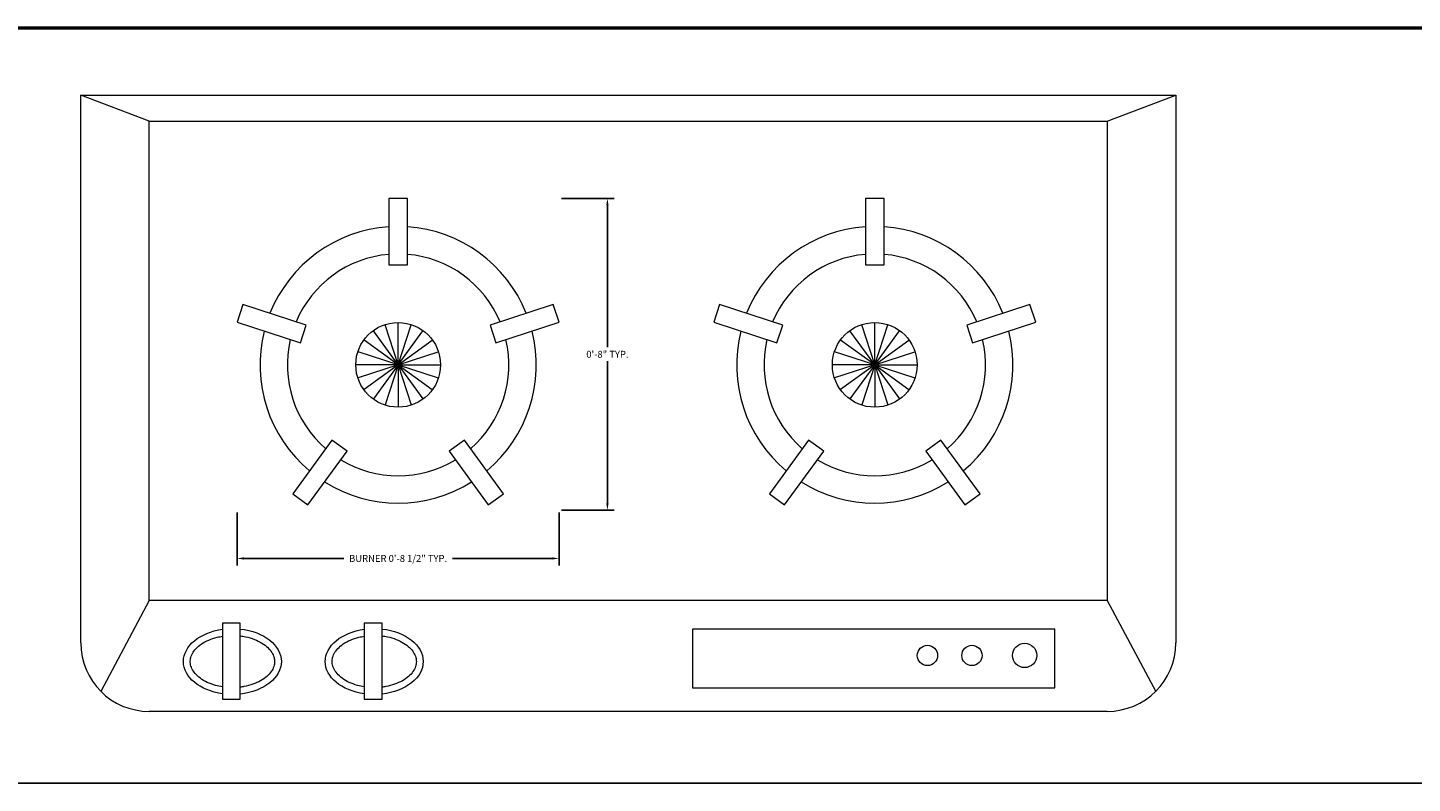
# Model space of a CAD drawing. Units: inches. Extents: x -173 to 545, y -746 to 104.
# Tile 28 of 32: x 189 to 225, y -12 to 8. Entities that reach past the tile are written whole.
import ezdxf

# ---------------------------------------------------------------- set-up
doc = ezdxf.new("R2010")
doc.units = ezdxf.units.IN
doc.header["$MEASUREMENT"] = 0
for name, color, linetype, lineweight in [('A-ANNO-DIMS', 2, 'Continuous', 18), ('A-EQPM', 8, 'Continuous', 18), ('A-FLOR-CASE', 9, 'Continuous', 25), ('A-WALL', 7, 'Continuous', 50)]:
    doc.layers.add(name, color=color, linetype=linetype, lineweight=lineweight)
doc.styles.get("Standard").update_dxf_attribs({"font": 'arial.ttf'})
doc.dimstyles.get("Standard").update_dxf_attribs({"dimtxt": 0.18, "dimasz": 0.18, "dimexe": 0.18, "dimexo": 0.0625, "dimgap": 0.09, "dimtad": 0, "dimtih": 1, "dimtoh": 1, "dimdec": 0, "dimzin": 0, "dimdsep": 46, "dimlunit": 3, "dimtxsty": 'Standard', "dimcen": 0.09, "dimadec": 0, "dimazin": 0, "dimtfac": 1, "dimtdec": 0, "dimtofl": 0, "dimtmove": 0, "dimatfit": 3, "dimfxl": 1, "dimtolj": 1, "dimtzin": 0, "dimarcsym": 0})

# ---------------------------------------------------------------- blocks, each defined once
blk = doc.blocks.new('HOB-28-BURNER')
for p, q in [((4.43, 7.964), (3.944, 7.964)), ((3.944, 7.964), (3.944, 6.235)), ((4.43, 6.235), (4.43, 7.964)), ((3.944, 6.235), (4.43, 6.235)), ((0.151, 5.207), (0, 4.745)), ((1.795, 4.673), (0.151, 5.207)), ((8.223, 5.207), (6.579, 4.673)), ((8.374, 4.745), (8.223, 5.207)), ((0, 4.745), (1.644, 4.211)), ((4.187, 3.64), (3.848, 4.683)), ((4.187, 3.64), (4.187, 4.737)), ((4.187, 3.64), (4.526, 4.683)), ((6.73, 4.211), (8.374, 4.745)), ((1.644, 4.211), (1.795, 4.673)), ((4.187, 3.64), (3.543, 4.527)), ((4.187, 3.64), (4.831, 4.527)), ((6.579, 4.673), (6.73, 4.211)), ((4.187, 3.64), (3.144, 3.979)), ((4.187, 3.64), (3.3, 4.285)), ((4.187, 3.64), (5.074, 4.285)), ((4.187, 3.64), (5.23, 3.979)), ((4.187, 3.64), (3.091, 3.64)), ((4.187, 3.64), (3.144, 3.302)), ((4.187, 3.64), (3.3, 2.996)), ((4.187, 3.64), (3.543, 2.754)), ((4.187, 3.64), (3.848, 2.598)), ((4.187, 3.64), (4.187, 2.544)), ((4.187, 3.64), (4.526, 2.598)), ((4.187, 3.64), (4.831, 2.754)), ((4.187, 3.64), (5.074, 2.996)), ((4.187, 3.64), (5.23, 3.302)), ((4.187, 3.64), (5.283, 3.64)), ((2.465, 1.684), (1.449, 0.286)), ((2.859, 1.399), (2.465, 1.684)), ((5.909, 1.684), (5.515, 1.399)), ((6.925, 0.286), (5.909, 1.684)), ((1.842, 0), (2.859, 1.399)), ((5.515, 1.399), (6.532, 0)), ((1.449, 0.286), (1.842, 0)), ((6.532, 0), (6.925, 0.286))]:
    blk.add_line(p, q)
blk.add_circle((4.187, 3.64), 1.101)
for radius, start, end in [(3.593, 93.8765, 158.1235), (3.593, 21.8765, 86.1235), (2.881, 94.8365, 157.1635), (2.881, 22.8365, 85.1635), (3.593, 165.8765, 230.1235), (3.593, 309.8765, 14.1235), (2.881, 166.8365, 229.1635), (2.881, 310.8365, 13.1635), (2.881, 238.8365, 301.1635), (3.593, 237.8765, 302.1235)]:
    blk.add_arc((4.187, 3.64), radius, start, end)
blk = doc.blocks.new('COUNTER-L-RETURN')
blk.add_line((66, 69.362), (0, 69.362))
blk = doc.blocks.new('*D70')
at = {"layer": 'A-ANNO-DIMS', "color": 0, "lineweight": -2, "transparency": 16777216}
for p, q in [((194.228, -4.963), (194.228, -6.336)), ((202.602, -4.963), (202.602, -6.336)), ((194.408, -6.156), (197.005, -6.156)), ((202.422, -6.156), (199.825, -6.156))]:
    blk.add_line(p, q, dxfattribs=at)
at = {"layer": 'A-ANNO-DIMS', "color": 0, "transparency": 16777216}
for points in [[(194.408, -6.126), (194.408, -6.186), (194.228, -6.156)], [(202.422, -6.126), (202.422, -6.186), (202.602, -6.156)]]:
    blk.add_solid(points, dxfattribs=at)
at = {"layer": 'Defpoints', "color": 0, "transparency": 16777216}
for p in [(194.228, -4.9), (202.602, -4.9), (202.602, -6.156)]:
    blk.add_point(p, dxfattribs=at)
at = {"layer": 'A-ANNO-DIMS', "color": 0, "transparency": 16777216, "insert": (198.415, -6.156), "char_height": 0.18, "attachment_point": 5}
blk.add_mtext('\\A1;BURNER 0\'-8 1/2" TYP.', dxfattribs=at)
blk = doc.blocks.new('*D71')
at = {"layer": 'A-ANNO-DIMS', "color": 0, "lineweight": -2, "transparency": 16777216}
for p, q in [((202.664, 3.2), (204.038, 3.2)), ((203.858, 3.02), (203.858, -0.668)), ((203.858, -4.72), (203.858, -1.032)), ((202.664, -4.9), (204.038, -4.9))]:
    blk.add_line(p, q, dxfattribs=at)
at = {"layer": 'A-ANNO-DIMS', "color": 0, "transparency": 16777216}
for points in [[(203.828, 3.02), (203.888, 3.02), (203.858, 3.2)], [(203.828, -4.72), (203.888, -4.72), (203.858, -4.9)]]:
    blk.add_solid(points, dxfattribs=at)
at = {"layer": 'Defpoints', "color": 0, "transparency": 16777216}
for p in [(202.602, 3.2), (203.858, 3.2), (202.602, -4.9)]:
    blk.add_point(p, dxfattribs=at)
at = {"layer": 'A-ANNO-DIMS', "color": 0, "transparency": 16777216, "insert": (203.858, -0.85), "char_height": 0.18, "attachment_point": 5}
blk.add_mtext('\\A1;0\'-8" TYP.', dxfattribs=at)

msp = doc.modelspace()

# ---------------------------------------------------------------- linework, layer by layer
at = {"layer": 'A-EQPM'}
for p, q in [((190.161, -8.351), (190.161, 5.888)), ((190.161, 5.888), (218.638, 5.888)), ((191.941, 5.211), (190.161, 5.888)), ((216.859, 5.211), (218.638, 5.888)), ((218.638, 5.888), (218.638, -8.351)), ((191.941, -7.248), (191.941, 5.211)), ((191.941, 5.211), (216.859, 5.211)), ((216.859, 5.211), (216.859, -7.248)), ((191.941, -7.248), (190.682, -9.61)), ((216.859, -7.248), (191.941, -7.248)), ((216.859, -7.248), (218.117, -9.61)), ((194.309, -7.842), (193.848, -7.842)), ((193.848, -7.842), (193.848, -9.811)), ((194.309, -9.811), (194.309, -7.842)), ((197.535, -7.842), (197.535, -9.811)), ((197.996, -7.842), (197.535, -7.842)), ((197.996, -9.811), (197.996, -7.842)), ((215.498, -7.993), (206.075, -7.993)), ((206.075, -7.993), (206.075, -9.519)), ((215.498, -9.519), (215.498, -7.993)), ((206.075, -9.519), (215.498, -9.519)), ((193.848, -9.811), (194.309, -9.811)), ((197.535, -9.811), (197.996, -9.811)), ((216.859, -10.131), (191.941, -10.131))]:
    msp.add_line(p, q, dxfattribs=at)
for centre, radius in [((212.181, -8.677), 0.263), ((213.339, -8.677), 0.263), ((214.708, -8.677), 0.316)]:
    msp.add_circle(centre, radius, dxfattribs=at)
for centre, start, end in [((191.941, -8.351), 180, 270), ((216.859, -8.351), 270, 0)]:
    msp.add_arc(centre, 1.78, start, end, dxfattribs=at)
at = {"layer": 'A-EQPM', "extrusion": (0, 0, -1)}
for centre, major_axis, start_param, end_param in [((194.106, -8.835), (1.274, 0), 1.774361, 4.508825), ((194.106, -8.835), (-1.274, 0), 1.73081, 4.552375), ((197.793, -8.835), (1.274, 0), 1.774361, 4.508825), ((197.793, -8.835), (-1.274, 0), 1.73081, 4.552375)]:
    msp.add_ellipse(centre, major_axis=major_axis, ratio=0.671641, start_param=start_param, end_param=end_param, dxfattribs=at)
at = {"layer": 'A-EQPM'}
for points, knots in [([(193.848, -9.493), (193.786, -9.484), (193.725, -9.471), (193.59, -9.433), (193.518, -9.407), (193.385, -9.345), (193.325, -9.309), (193.22, -9.232), (193.175, -9.191), (193.101, -9.105), (193.073, -9.061), (193.032, -8.974), (193.019, -8.931), (193.007, -8.845), (193.009, -8.802), (193.025, -8.716), (193.041, -8.672), (193.088, -8.585), (193.119, -8.541), (193.199, -8.457), (193.247, -8.416), (193.358, -8.342), (193.421, -8.308), (193.558, -8.249), (193.632, -8.224), (193.755, -8.194), (193.801, -8.184), (193.848, -8.177)], [8.079302, 8.079302, 8.079302, 8.079302, 8.245651, 8.245651, 8.463703, 8.463703, 8.681755, 8.681755, 8.899807, 8.899807, 9.117859, 9.117859, 9.33591, 9.33591, 9.553962, 9.553962, 9.772014, 9.772014, 9.990066, 9.990066, 10.208118, 10.208118, 10.426169, 10.426169, 10.644221, 10.644221, 10.770253, 10.770253, 10.770253, 10.770253]), ([(194.309, -8.17), (194.356, -8.175), (194.403, -8.183), (194.528, -8.209), (194.605, -8.232), (194.747, -8.286), (194.812, -8.319), (194.929, -8.39), (194.981, -8.43), (195.068, -8.513), (195.103, -8.556), (195.157, -8.643), (195.176, -8.687), (195.197, -8.765), (195.202, -8.8), (195.202, -8.835), (195.202, -8.878), (195.195, -8.921), (195.166, -9.008), (195.144, -9.052), (195.084, -9.139), (195.046, -9.181), (194.953, -9.263), (194.899, -9.301), (194.776, -9.37), (194.709, -9.401), (194.563, -9.452), (194.485, -9.472), (194.373, -9.492), (194.341, -9.497), (194.309, -9.501)], [4.889299, 4.889299, 4.889299, 4.889299, 5.015191, 5.015191, 5.233243, 5.233243, 5.451295, 5.451295, 5.669347, 5.669347, 5.887399, 5.887399, 6.10545, 6.10545, 6.283185, 6.283185, 6.283185, 6.501237, 6.501237, 6.719289, 6.719289, 6.937341, 6.937341, 7.155392, 7.155392, 7.373444, 7.373444, 7.591496, 7.591496, 7.677072, 7.677072, 7.677072, 7.677072]), ([(197.535, -9.493), (197.473, -9.484), (197.413, -9.471), (197.278, -9.433), (197.205, -9.407), (197.073, -9.345), (197.012, -9.309), (196.907, -9.232), (196.862, -9.191), (196.789, -9.105), (196.76, -9.061), (196.719, -8.974), (196.706, -8.931), (196.695, -8.845), (196.696, -8.802), (196.713, -8.716), (196.728, -8.672), (196.775, -8.585), (196.807, -8.541), (196.886, -8.457), (196.934, -8.416), (197.045, -8.342), (197.108, -8.308), (197.245, -8.249), (197.319, -8.224), (197.442, -8.194), (197.488, -8.184), (197.535, -8.177)], [8.079302, 8.079302, 8.079302, 8.079302, 8.245651, 8.245651, 8.463703, 8.463703, 8.681755, 8.681755, 8.899807, 8.899807, 9.117859, 9.117859, 9.33591, 9.33591, 9.553962, 9.553962, 9.772014, 9.772014, 9.990066, 9.990066, 10.208118, 10.208118, 10.426169, 10.426169, 10.644221, 10.644221, 10.770253, 10.770253, 10.770253, 10.770253]), ([(197.996, -8.17), (198.044, -8.175), (198.091, -8.183), (198.216, -8.209), (198.292, -8.232), (198.434, -8.286), (198.5, -8.319), (198.617, -8.39), (198.668, -8.43), (198.755, -8.513), (198.79, -8.556), (198.845, -8.643), (198.863, -8.687), (198.884, -8.765), (198.889, -8.8), (198.889, -8.835), (198.889, -8.878), (198.882, -8.921), (198.854, -9.008), (198.832, -9.052), (198.771, -9.139), (198.733, -9.181), (198.64, -9.263), (198.586, -9.301), (198.464, -9.37), (198.396, -9.401), (198.25, -9.452), (198.173, -9.472), (198.06, -9.492), (198.028, -9.497), (197.996, -9.501)], [4.889299, 4.889299, 4.889299, 4.889299, 5.015191, 5.015191, 5.233243, 5.233243, 5.451295, 5.451295, 5.669347, 5.669347, 5.887399, 5.887399, 6.10545, 6.10545, 6.283185, 6.283185, 6.283185, 6.501237, 6.501237, 6.719289, 6.719289, 6.937341, 6.937341, 7.155392, 7.155392, 7.373444, 7.373444, 7.591496, 7.591496, 7.677072, 7.677072, 7.677072, 7.677072])]:
    msp.add_open_spline(points, degree=3, knots=knots, dxfattribs=at)
at = {"layer": 'A-WALL'}
msp.add_line((169.801, 7.638), (260.801, 7.638), dxfattribs=at)

# ---------------------------------------------------------------- block references
at = {"layer": 'A-EQPM'}
for p in [(194.228, -4.764), (206.624, -4.764)]:
    msp.add_blockref('HOB-28-BURNER', p, dxfattribs=at)
at = {"layer": 'A-FLOR-CASE'}
msp.add_blockref('COUNTER-L-RETURN', (169.801, -81.362), dxfattribs=at)

# ---------------------------------------------------------------- dimensions: what is measured, and where the dimension line sits
at = {"layer": 'A-ANNO-DIMS'}
dim = msp.add_linear_dim(base=(203.858, 3.2), p1=(202.602, -4.9), p2=(202.602, 3.2), angle=90, text='<> TYP.', dimstyle='Standard', override={"dimdec": 1, "dimlfac": 1, "dimrnd": 0, "dimzin": 1, "dimdsep": 46, "dimlunit": 4, "dimfrac": 2}, dxfattribs=at)
dim.commit()
dim.dimension.update_dxf_attribs({"geometry": '*D71', "text_midpoint": (203.858, -0.85)})
dim = msp.add_linear_dim(base=(202.602, -6.156), p1=(194.228, -4.9), p2=(202.602, -4.9), text='BURNER <> TYP.', dimstyle='Standard', override={"dimdec": 1, "dimlfac": 1, "dimrnd": 0, "dimzin": 1, "dimdsep": 46, "dimlunit": 4, "dimfrac": 2}, dxfattribs=at)
dim.commit()
dim.dimension.update_dxf_attribs({"geometry": '*D70', "text_midpoint": (198.415, -6.156)})

doc.saveas('drawing.dxf')
